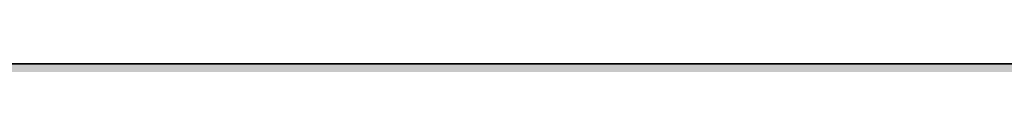
# Model space of a CAD drawing. Units: inches. Extents: x 2091 to 2899, y 967 to 2217.
# Tile 95 of 256: x 2251.5278 to 2251.8124, y 1099.9191 to 1099.9191. Entities that reach past the tile are written whole.
import ezdxf

# ---------------------------------------------------------------- set-up
doc = ezdxf.new("R2010")
doc.units = ezdxf.units.IN
doc.layers.add('A-WALL-PATT', color=141, linetype='Continuous', lineweight=13, true_color=0xadddf7)
doc.layers.add('L-SITE-WALL', color=7, linetype='Continuous', lineweight=35)

msp = doc.modelspace()

# ---------------------------------------------------------------- hatches: boundary and pattern name
at = {"layer": 'A-WALL-PATT'}
h = msp.add_hatch(color=256, dxfattribs=at)
h.dxf.hatch_style = 1
h.paths.add_polyline_path([(2212.1436, 1941.41906), (2387.6436, 1941.41906), (2387.6436, 1824.41906), (2392.1436, 1824.41906), (2392.1436, 1941.41906), (2609.6436, 1941.41906), (2609.6436, 1825.91906), (2614.1436, 1825.91906), (2614.1436, 1941.41906), (2794.1436, 1941.41906), (2794.1436, 1928.76217), (2803.1436, 1928.76217), (2803.1436, 2050.91906), (2203.1436, 2050.91906), (2203.1436, 1900.75786), (2212.1436, 1900.75786)])
h.paths.add_polyline_path([(2212.1436, 1945.91906), (2212.1436, 2041.91906), (2794.1436, 2041.91906), (2794.1436, 1945.91906), (2402.24824, 1945.91906), (2401.10243, 1945.77583), (2398.70243, 1945.77583)], flags=16)
h.paths.add_polyline_path([(2230.22986, 1948.06279), (2227.34986, 1949.50279), (2225.90986, 1951.90279), (2223.98986, 1952.86279), (2223.02986, 1955.26279), (2222.06986, 1959.58279), (2222.06986, 1963.42279), (2223.02986, 1965.66279), (2223.98986, 1965.34279), (2225.58591, 1963.86075), (2226.91153, 1964.95726), (2226.94886, 1965.93879), (2227.77832, 1966.95214), (2228.19992, 1968.8787), (2230.70986, 1964.86279), (2233.58986, 1966.30279), (2233.60731, 1966.33187), (2233.77266, 1964.9382), (2234.6338, 1963.67647), (2235.02986, 1963.90279), (2236.28203, 1965.57236), (2235.98986, 1962.94279), (2237.95451, 1957.54), (2238.38986, 1957.90279), (2239.21586, 1960.30579), (2238.65457, 1966.38496), (2238.69279, 1966.43807), (2238.84058, 1967.49971), (2238.78029, 1967.68749), (2238.88054, 1967.78676), (2238.66686, 1966.25179), (2239.21586, 1960.30579), (2238.38986, 1957.90279), (2236.94986, 1956.70279), (2234.54986, 1949.98279)], flags=0)
h.paths.add_polyline_path([(2278.01197, 1948.06279), (2276.49643, 1947.87335), (2275.84983, 1947.68861), (2274.65197, 1947.10279)], flags=0)
h.paths.add_polyline_path([(2269.85197, 1955.74279), (2268.27618, 1956.62933), (2270.8673, 1956.3484), (2269.37197, 1958.14279), (2268.71496, 1959.19233), (2270.56983, 1958.72861), (2268.58073, 1961.90609), (2270.81197, 1960.89188), (2270.81197, 1963.42279), (2271.39331, 1964.77926), (2270.29176, 1966.1562), (2271.77197, 1965.66279), (2272.14139, 1966.52476), (2273.92983, 1965.92861), (2275.63039, 1968.0543), (2276.33194, 1966.72186), (2276.52043, 1966.95214), (2276.94203, 1968.8787), (2277.73429, 1967.61108), (2278.13989, 1969.46452), (2279.65912, 1967.03374), (2280.41197, 1966.78279), (2280.9493, 1967.58879), (2281.60983, 1967.36861), (2282.13327, 1968.15376), (2282.34924, 1966.33344), (2282.34985, 1966.33259), (2283.40755, 1968.09542), (2283.71263, 1965.52402), (2284.32022, 1964.63379), (2284.51181, 1964.88924), (2284.23497, 1965.70479), (2284.50047, 1967.31896), (2284.90794, 1965.41742), (2285.39631, 1966.06858), (2285.43283, 1966.29061), (2285.47334, 1966.17128), (2286.35392, 1967.34539), (2286.22201, 1966.15817), (2287.66349, 1968.08015), (2287.71397, 1968.44279), (2288.4816, 1969.01668), (2288.57399, 1968.7289), (2288.91746, 1969.06904), (2288.60683, 1966.83761), (2288.92873, 1963.35131), (2288.93497, 1963.35679), (2288.92973, 1963.34042), (2289.01528, 1962.41387), (2290.11122, 1963.87513), (2290.13283, 1963.94261), (2290.21767, 1964.01706), (2290.11122, 1963.87513), (2289.15583, 1960.89161), (2288.59404, 1959.25723), (2288.57197, 1959.10279), (2289.53197, 1960.54279), (2290.01197, 1962.46279), (2290.19184, 1962.64266), (2289.76983, 1959.68861), (2286.88983, 1957.28861), (2284.48983, 1950.56861), (2283.31466, 1950.04631), (2283.29197, 1949.98279), (2280.29006, 1948.64861), (2281.12983, 1948.64861), (2282.56983, 1948.16861), (2283.20473, 1948.06279), (2278.97197, 1948.06279), (2276.09197, 1949.50279), (2274.65197, 1951.90279), (2272.73197, 1952.86279)], flags=0)
h.paths.add_polyline_path([(2271.15887, 1958.02177), (2272.96983, 1955.84861), (2272.00983, 1960.16861), (2272.00983, 1964.00861), (2272.62443, 1965.44266), (2274.32802, 1963.86075), (2275.65365, 1964.95726), (2275.63774, 1964.53909), (2277.41223, 1966.00689), (2277.03297, 1965.15679), (2276.82992, 1964.9756), (2276.76601, 1963.29501), (2277.44964, 1962.66022), (2279.45197, 1964.86279), (2282.33197, 1966.30279), (2283.52983, 1966.88861), (2283.29451, 1966.77095), (2283.91299, 1963.8847), (2284.89925, 1964.44827), (2284.73197, 1962.94279), (2286.69662, 1957.54), (2287.13197, 1957.90279), (2287.54191, 1959.09539), (2287.7794, 1958.44231), (2285.68274, 1956.6951), (2285.8765, 1959.79534), (2284.73197, 1962.94279), (2284.89925, 1964.44827), (2283.91299, 1963.8847), (2284.22383, 1962.43412), (2283.42436, 1963.60548), (2281.60983, 1962.56861), (2281.12983, 1960.16861), (2282.08983, 1956.32861), (2283.04983, 1952.96861), (2282.56983, 1950.56861), (2280.16983, 1948.64861), (2279.88332, 1948.79187), (2278.97197, 1948.06279), (2278.97197, 1949.02279), (2278.67231, 1949.39737), (2277.28983, 1950.08861), (2275.84983, 1952.48861), (2273.92983, 1953.44861), (2272.48983, 1954.88861), (2271.92165, 1954.88861), (2271.77197, 1955.26279)], flags=0)
h.paths.add_polyline_path([(2311.99415, 1955.74279), (2312.06272, 1955.67422), (2312.0551, 1955.7085)], flags=0)
h.paths.add_polyline_path([(2331.95615, 1963.95179), (2333.39615, 1965.39179), (2331.07715, 1963.35679), (2330.9986, 1963.11152)], flags=0)
h.paths.add_polyline_path([(2310.55415, 1954.30279), (2307.03981, 1956.27994), (2310.7629, 1955.87628), (2312.47415, 1953.82279), (2313.43415, 1951.42279), (2315.35415, 1950.46279), (2316.79415, 1948.06279), (2317.46615, 1947.72679), (2319.36869, 1947.96461), (2317.75415, 1949.98279), (2317.56953, 1950.61048), (2316.79415, 1951.90279), (2314.87415, 1952.86279), (2313.91415, 1955.26279), (2311.51415, 1958.14279), (2309.37549, 1961.55917), (2311.51415, 1960.33708), (2311.51415, 1961.98279), (2310.60467, 1963.11963), (2311.72661, 1962.47853), (2312.41833, 1964.09256), (2312.25596, 1964.29552), (2313.19415, 1963.98279), (2313.91415, 1965.66279), (2314.64678, 1965.41858), (2315.35415, 1966.30279), (2316.79415, 1967.74279), (2316.15744, 1966.9469), (2317.03411, 1965.28186), (2317.2226, 1965.51214), (2317.77705, 1968.04577), (2318.47411, 1966.72186), (2318.6626, 1966.95214), (2319.0842, 1968.8787), (2321.20705, 1965.48215), (2322.16142, 1966.9137), (2322.55415, 1966.78279), (2322.78599, 1967.13056), (2322.88165, 1966.32429), (2323.31204, 1965.72174), (2323.65129, 1965.89136), (2324.3965, 1967.13338), (2324.65694, 1964.9382), (2324.97199, 1964.47661), (2325.38728, 1967.0015), (2325.94081, 1964.41835), (2327.22893, 1966.13584), (2327.16632, 1965.57236), (2328.05914, 1966.76278), (2328.22458, 1966.24749), (2329.66797, 1967.67691), (2329.66458, 1967.68749), (2329.76482, 1967.78676), (2329.55115, 1966.25179), (2330.10015, 1960.30579), (2329.33281, 1958.07347), (2329.31306, 1957.93523), (2329.63415, 1958.20279), (2330.23415, 1959.10279), (2330.71415, 1961.02279), (2331.03415, 1961.34279), (2330.71415, 1959.10279), (2329.63415, 1958.20279), (2329.27415, 1957.66279), (2327.71211, 1956.3611), (2325.43415, 1949.98279), (2324.33377, 1949.49374), (2323.99415, 1948.54279), (2319.67415, 1946.62279), (2316.79415, 1948.06279), (2315.35415, 1950.46279), (2313.43415, 1951.42279)], flags=0)
h.paths.add_polyline_path([(2321.33568, 1947.95202), (2321.11415, 1948.06279), (2321.11415, 1949.02279), (2319.19415, 1951.42279), (2316.79415, 1959.58279), (2316.66324, 1959.58279), (2315.35415, 1958.14279), (2314.39415, 1958.14279), (2313.1483, 1958.70908), (2312.95415, 1959.58279), (2312.95415, 1960.89188), (2315.83415, 1959.58279), (2316.66324, 1959.58279), (2317.31471, 1960.29941), (2315.0302, 1962.42075), (2316.35582, 1963.51726), (2316.37234, 1963.95162), (2316.4702, 1963.86075), (2317.79582, 1964.95726), (2317.75522, 1963.88969), (2319.17515, 1965.15679), (2319.49841, 1965.88137), (2321.11415, 1965.34279), (2323.23589, 1962.37236), (2325.68635, 1963.77262), (2325.54279, 1962.48058), (2325.19878, 1963.49401), (2324.47851, 1963.08243), (2324.92601, 1960.99412), (2324.07809, 1962.23647), (2322.41479, 1961.28602), (2322.07415, 1959.58279), (2323.03415, 1955.74279), (2323.99415, 1952.38279), (2323.51415, 1949.98279), (2322.14272, 1948.88565), (2322.07415, 1948.54279)], flags=0)
h.paths.add_polyline_path([(2320.20748, 1963.33746), (2320.15415, 1963.42279), (2320.39415, 1963.54279)], flags=0)
h.paths.add_polyline_path([(2353.85053, 1965.8105), (2354.03053, 1965.7505), (2354.33053, 1966.4505), (2354.33053, 1966.9305)], flags=0)
h.paths.add_polyline_path([(2359.02058, 1969.02641), (2359.09838, 1968.90193), (2359.23353, 1969.5195), (2359.23353, 1969.9995)], flags=0)
h.paths.add_polyline_path([(2358.25669, 1966.68167), (2357.9836, 1966.34803), (2358.21127, 1966.14617), (2358.41049, 1966.38957)], flags=0)
h.paths.add_polyline_path([(2357.76847, 1966.05878), (2357.7322, 1965.10497), (2357.75105, 1965.12056), (2357.76953, 1965.6065), (2357.76953, 1966.05784)], flags=0)
h.paths.add_polyline_path([(2359.11153, 1965.3045), (2359.11153, 1964.8245), (2359.84453, 1966.4675), (2359.84453, 1966.9475)], flags=0)
h.paths.add_polyline_path([(2360.22368, 1966.62145), (2360.69853, 1969.3625), (2360.69853, 1969.8425), (2360.21053, 1967.0255), (2360.21053, 1966.6425)], flags=0)
h.paths.add_polyline_path([(2363.45053, 1967.8905), (2363.45053, 1968.3705), (2362.49053, 1966.9305), (2362.65604, 1966.69878)], flags=0)
h.paths.add_polyline_path([(2364.47552, 1966.07883), (2365.85053, 1968.3705), (2365.85053, 1968.8505), (2364.42798, 1966.47958)], flags=0)
h.paths.add_polyline_path([(2366.31353, 1965.8525), (2366.36671, 1965.69583), (2366.80253, 1968.3455), (2366.80253, 1968.8255)], flags=0)
h.paths.add_polyline_path([(2367.16531, 1965.80354), (2367.29053, 1966.9305), (2367.29053, 1967.4105), (2367.1027, 1965.72007)], flags=0)
h.paths.add_polyline_path([(2370.03653, 1959.9735), (2371.01353, 1963.0245), (2371.01353, 1963.5045), (2370.03653, 1960.4535)], flags=0)
h.paths.add_polyline_path([(2371.61053, 1960.2105), (2372.57053, 1961.6505), (2372.57053, 1962.1305), (2371.80253, 1960.9785)], flags=0)
h.paths.add_polyline_path([(2350.87367, 1956.00509), (2351.93053, 1955.8905), (2354.49053, 1953.3305), (2353.85053, 1954.9305), (2351.45053, 1957.8105), (2347.93553, 1963.4255), (2347.93553, 1963.9055), (2351.45053, 1958.2905), (2353.70507, 1955.58505), (2352.89053, 1959.2505), (2352.89053, 1959.7305), (2352.89053, 1961.92479), (2356.73053, 1959.7305), (2358.45447, 1961.62684), (2354.81053, 1965.0105), (2355.03086, 1965.28591), (2358.69109, 1961.88712), (2361.53053, 1965.0105), (2364.3765, 1966.43348), (2364.52439, 1965.18691), (2365.45447, 1963.82418), (2365.88107, 1964.06795), (2365.37053, 1966.4505), (2365.37053, 1966.9305), (2366.81053, 1960.2105), (2366.81053, 1959.7305), (2366.38871, 1952.98141), (2367.77053, 1956.8505), (2368.64123, 1957.57608), (2366.81053, 1962.6105), (2366.81053, 1963.0905), (2368.77518, 1957.68771), (2369.21053, 1958.0505), (2370.00159, 1960.35187), (2369.47523, 1966.05267), (2369.51346, 1966.10578), (2369.51417, 1966.11091), (2369.47523, 1966.53267), (2369.51346, 1966.58578), (2369.61463, 1967.31259), (2369.18253, 1968.6585), (2369.18253, 1969.1385), (2369.60096, 1967.83519), (2369.7012, 1967.93447), (2369.71795, 1968.05474), (2370.14518, 1968.37414), (2369.77871, 1968.01122), (2369.7012, 1967.45447), (2370.46816, 1968.214), (2369.67494, 1967.26577), (2369.51417, 1966.11091), (2370.03653, 1960.4535), (2370.03653, 1959.9735), (2369.44176, 1958.24319), (2370.65053, 1959.2505), (2371.04582, 1962.01756), (2371.13053, 1962.1305), (2370.65053, 1958.7705), (2367.77053, 1956.3705), (2365.37053, 1949.6505), (2362.0791, 1948.18764), (2363.45053, 1947.7305), (2361.05053, 1947.7305), (2360.09053, 1947.7305), (2357.10386, 1947.35717), (2360.09053, 1948.2105), (2358.17053, 1949.1705), (2356.73053, 1951.5705), (2354.81053, 1952.5305), (2351.93053, 1955.4105)], flags=0)
h.paths.add_polyline_path([(2361.05053, 1948.6905), (2359.13053, 1951.0905), (2356.73053, 1959.2505), (2355.77053, 1959.2505), (2352.89053, 1960.55959), (2352.89053, 1961.44479), (2355.89053, 1959.7305), (2356.73053, 1959.7305), (2356.83719, 1959.36783), (2361.53053, 1964.5305), (2363.24842, 1965.38945), (2364.92531, 1963.0418), (2362.49053, 1961.6505), (2362.06386, 1959.51717), (2362.97053, 1955.8905), (2363.93053, 1952.5305), (2363.93053, 1952.0505), (2363.45053, 1949.6505), (2361.05053, 1947.7305)], flags=0)
h.paths.add_polyline_path([(2359.13053, 1951.5705), (2359.29053, 1951.3705), (2361.05053, 1954.4505), (2361.05053, 1954.9305)], flags=0)
h.paths.add_polyline_path([(2357.21953, 1966.5455), (2356.79253, 1968.8145), (2356.79253, 1969.2945), (2357.21953, 1967.0255)], flags=0)
h.paths.add_polyline_path([(2361.05053, 1954.4505), (2361.53053, 1958.7705), (2361.53053, 1959.2505), (2361.05053, 1954.9305)], flags=0)
h.paths.add_polyline_path([(2402.54829, 1948.48608), (2402.30243, 1948.41583), (2402.59043, 1948.41583)], flags=0)
h.paths.add_polyline_path([(2394.14243, 1956.09583), (2395.68505, 1954.55321), (2396.7205, 1953.97068), (2396.06243, 1955.61583), (2395.24138, 1956.6011), (2395.8789, 1956.44171), (2395.10243, 1959.93583), (2395.10243, 1963.77583), (2396.06243, 1966.01583), (2397.02243, 1965.69583), (2398.61848, 1964.21379), (2399.94411, 1965.3103), (2399.98143, 1966.29183), (2400.81089, 1967.30518), (2401.23249, 1969.23174), (2403.53795, 1965.54301), (2403.94198, 1967.38932), (2404.70243, 1967.13583), (2405.46033, 1966.07478), (2406.62243, 1966.65583), (2406.63988, 1966.68491), (2406.80523, 1965.29124), (2406.92569, 1965.11475), (2407.34243, 1964.97583), (2407.87433, 1965.77367), (2408.1691, 1964.39805), (2409.31461, 1965.9254), (2409.21746, 1965.05105), (2409.44523, 1963.13124), (2410.30637, 1961.86951), (2410.70243, 1962.09583), (2411.44227, 1963.08228), (2411.16543, 1963.89783), (2411.61643, 1966.63976), (2411.72536, 1966.79111), (2411.87315, 1967.85275), (2411.81286, 1968.04053), (2411.91311, 1968.1398), (2411.69943, 1966.60483), (2412.24843, 1960.65883), (2413.22543, 1963.70983), (2414.3779, 1964.72116), (2414.51315, 1965.69275), (2414.45286, 1965.88053), (2414.55311, 1965.9798), (2414.3779, 1964.72116), (2414.51982, 1964.8457), (2414.36536, 1964.63111), (2414.33943, 1964.44483), (2414.88843, 1958.49883), (2414.06243, 1956.09583), (2412.62243, 1954.89583), (2410.17137, 1948.03285), (2410.01672, 1948.0844), (2405.90243, 1946.25583), (2405.90243, 1947.21583), (2405.20425, 1948.08856), (2404.22243, 1948.41583), (2403.26243, 1948.41583), (2400.38243, 1949.85583), (2399.66243, 1951.05583), (2397.98243, 1952.73583), (2397.02243, 1953.21583), (2395.68505, 1954.55321), (2392.65678, 1956.25691)], flags=0)
h.paths.add_polyline_path([(2409.08565, 1964.40744), (2409.13036, 1964.27572), (2409.26243, 1964.49583)], flags=0)
h.paths.add_polyline_path([(2397.74243, 1961.61583), (2398.70243, 1963.85583), (2399.66243, 1963.53583), (2401.42656, 1965.74099), (2401.79142, 1966.5588), (2402.07143, 1965.07083), (2402.83551, 1964.39337), (2403.2624, 1964.9149), (2403.33812, 1964.77109), (2402.61552, 1963.97622), (2402.49861, 1960.90224), (2403.543, 1959.93245), (2404.4132, 1960.88968), (2404.70243, 1962.33583), (2407.91635, 1964.17235), (2409.52021, 1961.92694), (2410.98708, 1957.89304), (2411.42243, 1958.25583), (2412.04796, 1960.07562), (2412.41034, 1959.07909), (2411.67562, 1958.46682), (2411.66243, 1958.25583), (2411.62607, 1958.42553), (2409.98243, 1957.05583), (2407.58243, 1950.33583), (2403.26243, 1948.41583), (2403.26243, 1949.37583), (2401.34243, 1951.77583), (2399.41651, 1958.32398), (2397.74243, 1959.08492), (2397.74243, 1959.97012), (2397.10243, 1960.33583), (2397.74243, 1960.04492)], flags=0)
h.paths.add_polyline_path([(2405.90243, 1952.97583), (2405.95043, 1953.40783), (2406.01672, 1953.17583)], flags=0)
h.paths.add_polyline_path([(2449.81778, 1967.11401), (2449.75232, 1967.13583), (2449.7937, 1967.0779)], flags=0)
h.paths.add_polyline_path([(2451.6977, 1966.61812), (2451.74089, 1966.69012), (2451.69205, 1966.6657)], flags=0)
h.paths.add_polyline_path([(2454.34363, 1965.73757), (2455.75232, 1967.61583), (2455.99232, 1968.09583), (2454.3645, 1965.9254)], flags=0)
h.paths.add_polyline_path([(2457.54732, 1968.86383), (2457.78732, 1969.34383), (2457.05432, 1968.79583), (2457.00762, 1968.46034)], flags=0)
h.paths.add_polyline_path([(2456.92178, 1967.85666), (2456.80224, 1968.22902), (2456.723, 1967.6598)], flags=0)
h.paths.add_polyline_path([(2457.30232, 1967.37683), (2457.54232, 1967.85683), (2456.81032, 1966.83983), (2456.74052, 1966.70022), (2456.74902, 1966.60811)], flags=0)
h.paths.add_polyline_path([(2458.27532, 1963.70983), (2458.15534, 1963.33515), (2460.35432, 1965.26483), (2460.59432, 1965.74483)], flags=0)
h.paths.add_polyline_path([(2458.39232, 1962.81583), (2458.36409, 1962.61819), (2459.59232, 1964.25583), (2459.83232, 1964.73583)], flags=0)
h.paths.add_polyline_path([(2459.35232, 1962.81583), (2459.27232, 1962.49583), (2460.07232, 1963.29583), (2460.31232, 1963.77583)], flags=0)
h.paths.add_polyline_path([(2458.68032, 1960.60783), (2458.63232, 1960.41583), (2459.59232, 1961.85583), (2459.83232, 1962.33583)], flags=0)
h.paths.add_polyline_path([(2437.83817, 1956.24265), (2439.19232, 1956.09583), (2441.35232, 1953.93583), (2440.87232, 1955.13583), (2438.47232, 1958.01583), (2438.07156, 1958.65602), (2438.71232, 1958.49583), (2440.6396, 1956.18311), (2439.91232, 1959.45583), (2439.91232, 1963.29583), (2441.35232, 1966.65583), (2441.59232, 1967.13583), (2441.11232, 1966.01583), (2442.07232, 1965.69583), (2443.98899, 1968.09167), (2444.24132, 1966.75083), (2444.9168, 1966.15192), (2445.67657, 1967.08014), (2446.25532, 1969.72483), (2446.49532, 1970.20483), (2446.28238, 1969.23174), (2447.36267, 1967.50327), (2447.72032, 1969.56783), (2447.96032, 1970.04783), (2447.48548, 1967.30678), (2448.79232, 1965.21583), (2448.47232, 1964.86383), (2448.55232, 1964.73583), (2451.45205, 1966.1857), (2451.61512, 1964.81124), (2452.30792, 1963.79617), (2453.23451, 1964.32565), (2454.07232, 1960.41583), (2453.62869, 1953.31765), (2454.79232, 1956.57583), (2455.03232, 1957.05583), (2455.71884, 1957.62793), (2453.83232, 1962.81583), (2453.94097, 1963.79362), (2453.33532, 1965.57783), (2453.82432, 1968.55083), (2454.06432, 1969.03083), (2453.57532, 1966.05783), (2454.04033, 1964.68792), (2453.83232, 1962.81583), (2455.71884, 1957.62793), (2456.36721, 1958.16824), (2457.05832, 1960.17883), (2457.29832, 1960.65883), (2456.47232, 1958.25583), (2457.71773, 1959.29367), (2457.67232, 1958.97583), (2454.88995, 1956.65719), (2453.61414, 1953.08492), (2453.59232, 1952.73583), (2453.35232, 1952.25583), (2453.3596, 1952.3722), (2452.63232, 1950.33583), (2452.39232, 1949.85583), (2449.20375, 1948.43869), (2450.71232, 1947.93583), (2448.07232, 1947.93583), (2447.11232, 1947.93583), (2444.55232, 1947.61583), (2447.1996, 1948.3722), (2445.19232, 1949.37583), (2443.75232, 1951.77583), (2441.83232, 1952.73583), (2438.95232, 1955.61583)], flags=0)
h.paths.add_polyline_path([(2443.99232, 1959.93583), (2444.04032, 1959.77263), (2444.12155, 1959.86199)], flags=0)
h.paths.add_polyline_path([(2442.91232, 1959.93583), (2443.03232, 1959.93583), (2442.44566, 1960.2025)], flags=0)
h.paths.add_polyline_path([(2444.98294, 1965.01968), (2445.27932, 1965.26483), (2445.51932, 1965.74483), (2444.994, 1965.3103)], flags=0)
h.paths.add_polyline_path([(2446.13332, 1965.02983), (2446.33037, 1965.4715), (2444.97032, 1964.25783), (2444.73032, 1963.77783)], flags=0)
h.paths.add_polyline_path([(2442.79232, 1959.45583), (2443.75232, 1959.45583), (2446.15232, 1951.29583), (2446.41232, 1951.75083), (2446.39232, 1951.77583), (2448.0806, 1954.73032), (2448.55232, 1958.97583), (2441.83232, 1965.21583), (2442.15495, 1965.61911), (2448.79232, 1959.45583), (2448.31232, 1955.13583), (2448.07232, 1954.65583), (2446.41232, 1951.75083), (2448.31232, 1949.37583), (2448.31232, 1948.41583), (2450.54089, 1950.19869), (2450.95232, 1952.25583), (2449.99232, 1955.61583), (2449.03232, 1959.45583), (2449.51232, 1961.85583), (2449.75232, 1962.33583), (2449.6749, 1961.94874), (2452.99451, 1963.84565), (2453.06441, 1963.51941), (2452.88461, 1963.78285), (2449.6749, 1961.94874), (2449.27232, 1959.93583), (2450.23232, 1956.09583), (2451.19232, 1952.73583), (2450.71232, 1950.33583), (2450.47232, 1949.85583), (2448.07232, 1947.93583), (2448.07232, 1948.53583), (2445.43232, 1949.85583), (2443.99232, 1952.25583), (2442.07232, 1953.21583), (2441.11232, 1955.61583), (2440.15232, 1959.93583), (2440.15232, 1960.65583)], flags=0)
h.paths.add_polyline_path([(2456.69232, 1966.98583), (2457.60832, 1968.08083), (2457.84832, 1968.56083), (2456.93232, 1967.46583)], flags=0)
h.paths.add_polyline_path([(2489.89657, 1966.58024), (2489.94295, 1966.18935), (2490.74749, 1967.53025), (2491.31912, 1968.95116)], flags=0)
h.paths.add_polyline_path([(2473.56247, 1956.40713), (2477.13998, 1956.01926), (2476.95533, 1956.24083), (2475.10805, 1957.28011), (2476.34749, 1956.97025), (2475.1869, 1958.82422), (2476.91912, 1958.39116), (2475.41164, 1960.79927), (2477.78749, 1959.71934), (2477.78749, 1962.25025), (2477.6374, 1962.43786), (2477.82255, 1962.33206), (2478.35912, 1963.58406), (2478.35912, 1963.67116), (2477.32435, 1964.96463), (2478.71483, 1964.50114), (2479.31912, 1965.91116), (2480.27912, 1965.59116), (2481.78397, 1967.47221), (2482.11649, 1965.70525), (2482.88056, 1965.02778), (2483.20931, 1965.42941), (2483.22017, 1965.71509), (2483.07594, 1965.98902), (2483.71176, 1966.76581), (2484.13049, 1968.67925), (2484.70212, 1970.10016), (2484.48918, 1969.12707), (2486.5029, 1965.90511), (2487.38749, 1965.61025), (2488.15342, 1966.75914), (2488.71702, 1965.97011), (2489.20009, 1966.21164), (2489.33067, 1965.11099), (2490.3939, 1963.62246), (2490.66077, 1963.77496), (2490.49391, 1964.55364), (2490.92306, 1963.92484), (2491.31912, 1964.15116), (2491.33339, 1964.17018), (2491.21049, 1964.53225), (2491.28176, 1964.96554), (2491.42579, 1964.29338), (2494.07648, 1967.82763), (2494.49792, 1966.51494), (2494.59817, 1966.61422), (2494.68949, 1967.27025), (2495.10675, 1967.5822), (2495.12984, 1967.74807), (2495.06955, 1967.93585), (2495.1698, 1968.03513), (2495.03178, 1967.04363), (2495.75382, 1967.75868), (2494.98205, 1966.68644), (2494.95612, 1966.50016), (2495.47902, 1960.83685), (2495.91049, 1962.18425), (2496.48212, 1963.60516), (2496.07269, 1962.32659), (2496.7689, 1962.93754), (2496.59912, 1962.71116), (2496.11912, 1959.35116), (2496.73287, 1960.27179), (2496.98749, 1961.29025), (2497.55912, 1962.71116), (2497.07912, 1960.79116), (2496.50749, 1959.37025), (2495.54749, 1957.93025), (2492.75884, 1955.60638), (2490.83912, 1950.23116), (2490.26749, 1948.81025), (2485.94749, 1946.89025), (2483.06749, 1948.33025), (2481.62749, 1950.73025), (2479.70749, 1951.69025), (2476.82749, 1954.57025)], flags=0)
h.paths.add_polyline_path([(2485.57697, 1948.31339), (2485.55912, 1948.31116), (2485.57876, 1948.31116)], flags=0)
h.paths.add_polyline_path([(2478.64506, 1954.55116), (2478.10904, 1956.96326), (2479.31912, 1955.51116), (2480.27912, 1953.11116), (2482.19912, 1952.15116), (2483.63912, 1949.75116), (2486.51912, 1948.31116), (2486.51912, 1949.27116), (2484.73931, 1951.49593), (2484.02749, 1950.25025), (2481.62749, 1958.41025), (2482.37515, 1959.23267), (2482.19912, 1959.83116), (2483.19757, 1960.92946), (2479.70749, 1964.17025), (2480.60336, 1965.29008), (2481.87517, 1964.10911), (2482.66639, 1964.76358), (2482.61536, 1963.4218), (2482.9892, 1963.07466), (2484.00849, 1963.98425), (2484.68361, 1965.49751), (2484.58012, 1965.40516), (2485.35727, 1967.14711), (2485.12065, 1965.7812), (2486.42749, 1963.69025), (2488.14538, 1964.5492), (2489.82227, 1962.20155), (2490.74749, 1962.73025), (2491.99966, 1964.39981), (2492.07605, 1965.08726), (2492.21289, 1964.68412), (2492.48537, 1965.04743), (2492.27912, 1963.19116), (2494.24377, 1957.78837), (2494.5625, 1958.05398), (2494.93349, 1959.13325), (2495.50512, 1960.55416), (2494.67912, 1958.15116), (2494.10749, 1956.73025), (2494.5625, 1958.05398), (2493.40854, 1957.09235), (2491.70749, 1961.77025), (2491.99966, 1964.39981), (2490.74749, 1962.73025), (2487.71203, 1960.9957), (2487.47912, 1959.83116), (2488.43912, 1955.99116), (2489.39912, 1952.63116), (2488.91912, 1950.23116), (2488.57692, 1949.9574), (2488.34749, 1948.81025), (2487.65172, 1948.25363), (2487.47912, 1948.31116), (2486.51912, 1948.31116), (2483.63912, 1949.75116), (2482.19912, 1952.15116), (2480.27912, 1953.11116), (2478.83912, 1954.55116)], flags=0)
h.paths.add_polyline_path([(2526.64825, 1966.98752), (2526.51734, 1967.03116), (2526.6001, 1966.9153)], flags=0)
h.paths.add_polyline_path([(2528.47064, 1966.44666), (2528.57449, 1966.61973), (2528.45707, 1966.56102)], flags=0)
h.paths.add_polyline_path([(2534.13334, 1967.49616), (2534.15669, 1967.54285), (2534.05984, 1967.4083)], flags=0)
h.paths.add_polyline_path([(2536.16192, 1964.0506), (2535.15734, 1962.71116), (2535.10087, 1962.31587), (2536.11734, 1963.67116), (2536.42053, 1964.27754)], flags=0)
h.paths.add_polyline_path([(2535.15734, 1959.83116), (2536.11734, 1961.27116), (2536.59734, 1962.23116), (2535.25334, 1960.21516)], flags=0)
h.paths.add_polyline_path([(2513.24904, 1956.2848), (2516.22118, 1955.96256), (2514.99734, 1957.43116), (2514.19582, 1958.71154), (2515.47734, 1958.39116), (2516.93189, 1956.64571), (2516.43734, 1958.87116), (2516.43734, 1962.71116), (2516.87269, 1963.72697), (2515.34643, 1965.6348), (2517.39734, 1964.95116), (2517.87734, 1966.07116), (2518.35734, 1967.03116), (2517.87734, 1965.91116), (2518.83734, 1965.59116), (2520.48659, 1967.65272), (2520.76634, 1966.16616), (2521.53042, 1965.48869), (2521.78144, 1965.79537), (2521.80091, 1966.30727), (2521.4778, 1966.92094), (2521.24634, 1967.12616), (2521.1777, 1967.49091), (2521.4778, 1966.92094), (2522.01042, 1966.44869), (2522.25739, 1966.75042), (2522.78034, 1969.14016), (2523.26034, 1970.10016), (2523.0474, 1969.12707), (2524.67313, 1966.5259), (2526.03734, 1966.07116), (2526.79524, 1965.01011), (2527.97707, 1965.60102), (2528.14014, 1964.22657), (2528.66459, 1963.45816), (2529.38862, 1963.87189), (2529.32967, 1964.14699), (2529.48128, 1963.92484), (2529.87734, 1964.15116), (2529.98401, 1964.29338), (2529.78905, 1965.20318), (2530.0624, 1964.3979), (2532.80248, 1968.05135), (2533.14777, 1966.97585), (2533.24802, 1967.07513), (2533.33934, 1967.73116), (2533.67285, 1967.98049), (2533.72802, 1968.03513), (2533.51434, 1966.50016), (2534.02472, 1960.9725), (2534.56034, 1962.64516), (2535.04034, 1963.60516), (2534.06334, 1960.55416), (2533.23734, 1958.15116), (2534.28815, 1959.02684), (2534.19734, 1958.39116), (2531.5126, 1956.15387), (2529.39734, 1950.23116), (2528.91734, 1949.27116), (2526.44877, 1948.17402), (2527.47734, 1947.83116), (2530.35734, 1947.35116), (2524.59734, 1947.35116), (2521.71734, 1948.79116), (2520.27734, 1951.19116), (2518.35734, 1952.15116), (2515.47734, 1955.03116)], flags=0)
h.paths.add_polyline_path([(2523.93476, 1967.19031), (2523.61951, 1966.48369), (2523.7705, 1966.24211)], flags=0)
h.paths.add_polyline_path([(2518.83734, 1953.11116), (2517.87734, 1955.51116), (2516.88498, 1959.97678), (2516.91734, 1959.96207), (2516.91734, 1962.02545), (2520.75734, 1959.83116), (2522.02495, 1961.22553), (2518.35734, 1964.63116), (2519.00259, 1965.43772), (2520.43339, 1964.10911), (2521.30112, 1964.82687), (2521.24516, 1963.35533), (2525.63831, 1959.27598), (2526.03734, 1961.27116), (2529.39734, 1963.19116), (2530.64952, 1964.86073), (2530.66472, 1964.99755), (2530.69196, 1964.91731), (2531.08778, 1965.44507), (2530.94599, 1964.16894), (2530.69196, 1964.91731), (2529.39734, 1963.19116), (2526.3625, 1961.45697), (2526.03734, 1959.83116), (2526.99734, 1955.99116), (2527.95734, 1952.63116), (2527.47734, 1950.23116), (2527.13449, 1949.95687), (2526.97393, 1949.15409), (2526.69734, 1949.03116), (2524.59734, 1947.35116), (2524.59734, 1948.31116), (2524.27734, 1948.71116), (2522.19734, 1949.75116), (2520.75734, 1952.15116)], flags=0)
h.paths.add_polyline_path([(2520.27734, 1958.87116), (2520.85334, 1959.50476), (2523.15734, 1951.67116), (2524.61389, 1954.22013), (2524.59734, 1954.07116), (2522.67734, 1950.71116)], flags=0)
h.paths.add_polyline_path([(2559.37091, 1966.31116), (2559.39841, 1966.32491), (2559.40194, 1966.3453)], flags=0)
h.paths.add_polyline_path([(2549.77091, 1957.19116), (2552.65091, 1954.31116), (2552.13399, 1955.60347), (2550.61091, 1957.43116), (2547.09591, 1963.04616), (2545.77591, 1965.20616), (2549.29091, 1959.59116), (2551.69091, 1956.71116), (2550.79293, 1960.75206), (2550.73091, 1960.78025), (2550.73091, 1964.87116), (2551.69091, 1967.11116), (2552.65091, 1966.79116), (2554.24696, 1965.30911), (2555.03425, 1965.96034), (2555.58167, 1966.64461), (2555.60991, 1967.38716), (2556.43937, 1968.40051), (2556.86097, 1970.32707), (2559.37091, 1966.31116), (2560.69091, 1964.15116), (2562.40881, 1965.01011), (2561.65091, 1966.07116), (2560.33091, 1968.23116), (2561.7585, 1966.23254), (2562.34721, 1967.11561), (2562.43371, 1966.38657), (2563.1278, 1965.3696), (2563.57091, 1965.59116), (2563.58836, 1965.62024), (2563.36254, 1967.52354), (2563.72249, 1965.84379), (2565.06, 1968.07298), (2564.73286, 1965.12872), (2565.11758, 1963.33338), (2567.44462, 1966.43611), (2567.31561, 1967.83333), (2567.35384, 1967.88644), (2567.50163, 1968.94807), (2567.44134, 1969.13585), (2567.54159, 1969.23513), (2567.32791, 1967.70016), (2567.87691, 1961.75416), (2568.74669, 1964.47033), (2568.63561, 1965.67333), (2568.67384, 1965.72644), (2568.82163, 1966.78807), (2568.76134, 1966.97585), (2568.86159, 1967.07513), (2568.64791, 1965.54016), (2568.72613, 1964.69303), (2568.85391, 1964.80516), (2568.74669, 1964.47033), (2568.81724, 1963.70626), (2568.97091, 1963.91116), (2568.86607, 1963.17731), (2569.19691, 1959.59416), (2568.37091, 1957.19116), (2566.93091, 1955.99116), (2564.62027, 1949.52137), (2564.65091, 1949.51116), (2564.61662, 1949.51116), (2564.53091, 1949.27116), (2560.21091, 1947.35116), (2557.33091, 1948.79116), (2556.0452, 1950.93402), (2556.01091, 1950.95116), (2555.85662, 1951.2083), (2553.97091, 1952.15116), (2551.09091, 1955.03116), (2546.65014, 1957.52951)], flags=0)
h.paths.add_polyline_path([(2567.02579, 1959.33023), (2567.03501, 1959.30489), (2567.05091, 1959.35116)], flags=0)
h.paths.add_polyline_path([(2551.96829, 1962.51837), (2553.01091, 1964.95116), (2553.97091, 1964.63116), (2555.56696, 1963.14911), (2556.89258, 1964.24563), (2556.92991, 1965.22716), (2557.14398, 1965.48869), (2556.42007, 1966.13056), (2556.39142, 1966.10499), (2556.37991, 1966.16616), (2556.42007, 1966.13056), (2556.95191, 1966.60516), (2557.09214, 1966.91948), (2557.57087, 1966.01023), (2557.75937, 1966.24051), (2557.41791, 1964.68016), (2556.89258, 1964.24563), (2556.80709, 1961.99757), (2560.69091, 1958.39116), (2560.63553, 1957.8927), (2560.81091, 1957.19116), (2561.77091, 1953.83116), (2561.29091, 1951.43116), (2559.11042, 1949.68677), (2559.15648, 1949.62919), (2563.02652, 1951.34921), (2562.61091, 1949.27116), (2560.21091, 1947.35116), (2560.21091, 1948.31116), (2559.25091, 1949.51116), (2558.89091, 1949.51116), (2558.89091, 1949.96116), (2558.29091, 1950.71116), (2558.0537, 1951.51767), (2556.97091, 1952.87116), (2555.06788, 1959.34146), (2552.05091, 1961.06545), (2552.05091, 1962.47116)], flags=0)
h.paths.add_polyline_path([(2588.33005, 1958.39116), (2588.61025, 1958.11096), (2588.55336, 1958.36695)], flags=0)
h.paths.add_polyline_path([(2594.74545, 1950.49309), (2593.95753, 1953.17202), (2593.13005, 1954.55116), (2591.21005, 1955.51116), (2590.25005, 1957.91116), (2588.30903, 1960.24038), (2586.17731, 1961.20935), (2587.85005, 1960.79116), (2587.25342, 1961.74425), (2588.44131, 1961.06545), (2588.44131, 1962.65553), (2588.42168, 1962.66535), (2588.44131, 1962.71116), (2586.91404, 1964.62026), (2588.87709, 1963.72796), (2589.29005, 1964.69154), (2589.29005, 1966.07116), (2590.25005, 1968.31116), (2591.21005, 1967.99116), (2592.8061, 1966.50911), (2594.13172, 1967.60563), (2594.16905, 1968.58716), (2594.99851, 1969.60051), (2595.4201, 1971.52707), (2597.93005, 1967.51116), (2600.81005, 1968.95116), (2600.8275, 1968.98024), (2600.99285, 1967.58657), (2601.85399, 1966.32484), (2602.10714, 1966.4695), (2602.23635, 1967.25507), (2602.35672, 1966.69338), (2603.50222, 1968.22073), (2603.21005, 1965.59116), (2605.1747, 1960.18837), (2605.50689, 1960.4652), (2605.02602, 1965.67333), (2605.06425, 1965.72644), (2605.21203, 1966.78807), (2605.15174, 1966.97585), (2605.25199, 1967.07513), (2605.34331, 1967.73116), (2605.9529, 1968.1869), (2605.87475, 1969.03333), (2605.91298, 1969.08644), (2606.06077, 1970.14807), (2606.00048, 1970.33585), (2606.10073, 1970.43513), (2605.88705, 1968.90016), (2606.43605, 1962.95416), (2605.61005, 1960.55116), (2605.99704, 1960.87365), (2606.56431, 1962.64516), (2608.24149, 1964.11694), (2608.01005, 1963.19116), (2607.05005, 1961.75116), (2606.63149, 1961.40236), (2606.20131, 1958.39116), (2603.32131, 1955.99116), (2600.92131, 1949.27116), (2596.60131, 1947.35116), (2593.72131, 1948.79116), (2592.85731, 1950.23116), (2592.65005, 1950.23116)], flags=0)
h.paths.add_polyline_path([(2596.60131, 1947.35116), (2596.60131, 1948.31116), (2594.68131, 1950.71116), (2596.15495, 1953.29003), (2595.53005, 1954.07116), (2593.19923, 1961.99596), (2592.65134, 1962.50471), (2591.78015, 1963.00253), (2593.28299, 1964.24563), (2593.32031, 1965.22716), (2594.14977, 1966.24051), (2594.57137, 1968.16707), (2596.18265, 1965.58902), (2596.95127, 1966.43451), (2598.04131, 1966.07116), (2598.79921, 1965.01011), (2599.96131, 1965.59116), (2599.97876, 1965.62024), (2600.14411, 1964.22657), (2601.00526, 1962.96484), (2601.40131, 1963.19116), (2602.65349, 1964.86073), (2602.36131, 1962.23116), (2603.79275, 1958.29472), (2601.97764, 1953.21243), (2601.94621, 1952.70945), (2599.46876, 1951.60836), (2599.00131, 1949.27116)], flags=0)
h.paths.add_polyline_path([(2597.56131, 1958.87116), (2597.67097, 1959.41942), (2597.59505, 1958.7362)], flags=0)
h.paths.add_polyline_path([(2623.6663, 1961.25438), (2625.51916, 1960.79116), (2624.96554, 1961.67553), (2627.19916, 1960.66025), (2627.19916, 1961.15116), (2626.95916, 1962.23116), (2626.95916, 1963.49116), (2625.58232, 1965.21221), (2626.95916, 1964.42545), (2626.95916, 1965.83116), (2626.86916, 1965.86116), (2627.91916, 1968.31116), (2628.87916, 1967.99116), (2630.47521, 1966.50911), (2631.80084, 1967.60563), (2631.83816, 1968.58716), (2632.66762, 1969.60051), (2633.08922, 1971.52707), (2635.59916, 1967.51116), (2638.47916, 1968.95116), (2638.49661, 1968.98024), (2638.66196, 1967.58657), (2639.17627, 1966.83301), (2639.78022, 1967.83958), (2640.02583, 1966.69338), (2641.17134, 1968.22073), (2640.87916, 1965.59116), (2641.11426, 1964.94463), (2641.41134, 1965.34073), (2641.3081, 1964.41159), (2642.84381, 1960.18837), (2643.27916, 1960.55116), (2644.08474, 1962.89474), (2643.78387, 1966.15333), (2643.80683, 1966.18524), (2643.60068, 1968.41805), (2643.52281, 1968.66058), (2643.72988, 1970.14807), (2643.66959, 1970.33585), (2643.76984, 1970.43513), (2643.55616, 1968.90016), (2643.60068, 1968.41805), (2643.90959, 1967.45585), (2644.00984, 1967.55513), (2643.81174, 1966.13208), (2644.10516, 1962.95416), (2644.23877, 1961.35084), (2644.71916, 1961.75116), (2645.03285, 1962.2217), (2645.32216, 1963.12516), (2646.07642, 1963.78705), (2645.03285, 1962.2217), (2644.34516, 1960.07416), (2643.51916, 1957.67116), (2642.07916, 1956.47116), (2639.71961, 1949.86442), (2639.87553, 1949.83843), (2635.35916, 1947.83116), (2632.47916, 1949.27116), (2631.03916, 1951.67116), (2629.11916, 1952.63116), (2628.15916, 1955.03116), (2625.75916, 1957.91116)], flags=0)
h.paths.add_polyline_path([(2627.81631, 1956.57402), (2627.37371, 1958.56571), (2626.37631, 1959.76259), (2627.19916, 1959.35116), (2627.37371, 1958.56571), (2627.91916, 1957.91116), (2628.87916, 1955.51116), (2630.79916, 1954.55116), (2632.23916, 1952.15116), (2633.31502, 1951.61323), (2631.03916, 1959.35116), (2631.49783, 1959.85569), (2630.79916, 1962.23116), (2631.44987, 1962.94694), (2630.71521, 1963.62911), (2632.04084, 1964.72563), (2632.07816, 1965.70716), (2632.29224, 1965.96869), (2631.70534, 1966.48907), (2633.13644, 1967.76614), (2633.32922, 1968.64707), (2634.67472, 1966.49427), (2635.20847, 1967.08139), (2636.79916, 1966.55116), (2637.6764, 1967.86702), (2638.99395, 1966.02246), (2639.70534, 1966.42898), (2641.11916, 1959.83116), (2640.93007, 1956.80571), (2639.43916, 1952.63116), (2638.22746, 1952.09262), (2637.75916, 1949.75116), (2635.35916, 1947.83116), (2635.35916, 1948.79116), (2633.43916, 1951.19116), (2633.31502, 1951.61323), (2632.23916, 1952.15116), (2630.79916, 1954.55116), (2628.87916, 1955.51116)], flags=0)
h.paths.add_polyline_path([(2637.75916, 1953.83116), (2637.27916, 1955.51116), (2636.31916, 1959.35116), (2636.79916, 1961.75116), (2639.23395, 1963.14246), (2637.55706, 1965.49011), (2638.73889, 1966.08102), (2638.90196, 1964.70657), (2639.7631, 1963.44484), (2636.79916, 1961.75116), (2636.5325, 1960.41783), (2637.03916, 1958.39116), (2637.99916, 1955.03116)], flags=0)
h.paths.add_polyline_path([(2668.56741, 1951.43116), (2667.60741, 1953.83116), (2665.20741, 1956.71116), (2662.2939, 1961.36531), (2665.44741, 1959.59116), (2666.64741, 1958.39116), (2666.64741, 1959.97516), (2666.05832, 1960.68207), (2666.64741, 1960.34545), (2666.64741, 1961.99116), (2666.70009, 1962.11409), (2666.40741, 1963.43116), (2666.40741, 1967.27116), (2667.36741, 1969.51116), (2668.32741, 1969.19116), (2669.92346, 1967.70911), (2671.24908, 1968.80563), (2671.28641, 1969.78716), (2672.11587, 1970.80051), (2672.53746, 1972.72707), (2675.04741, 1968.71116), (2677.92741, 1970.15116), (2677.94486, 1970.18024), (2678.11021, 1968.78657), (2678.97135, 1967.52484), (2679.36741, 1967.75116), (2680.61958, 1969.42073), (2680.32741, 1966.79116), (2682.29206, 1961.38837), (2682.72741, 1961.75116), (2683.35831, 1963.58657), (2683.23211, 1964.95333), (2683.27034, 1965.00644), (2683.39322, 1965.88914), (2683.35997, 1966.24921), (2683.35784, 1966.25585), (2683.35923, 1966.25723), (2682.99211, 1970.23333), (2683.03034, 1970.28644), (2683.17812, 1971.34807), (2683.11784, 1971.53585), (2683.21808, 1971.63513), (2683.00441, 1970.10016), (2683.35923, 1966.25723), (2683.45808, 1966.35513), (2683.39322, 1965.88914), (2683.41391, 1965.66502), (2684.42381, 1966.87227), (2683.55341, 1964.15416), (2683.35831, 1963.58657), (2683.79341, 1958.87416), (2682.96741, 1956.47116), (2681.52741, 1955.27116), (2680.10923, 1951.30025), (2680.08493, 1950.91157), (2679.97685, 1950.92959), (2679.12741, 1948.55116), (2674.80741, 1946.63116), (2671.92741, 1948.07116), (2670.48741, 1950.47116)], flags=0)
h.paths.add_polyline_path([(2671.93568, 1953.22702), (2671.68741, 1953.35116), (2670.24741, 1955.75116), (2668.32741, 1956.71116), (2667.35674, 1959.13783), (2669.52741, 1958.15116), (2670.48741, 1958.15116), (2671.47941, 1959.24236), (2670.6844, 1961.94538), (2668.8896, 1963.61198), (2667.30741, 1964.33116), (2668.56741, 1963.91116), (2668.83094, 1964.24057), (2670.24741, 1963.43116), (2672.42214, 1965.82337), (2672.77746, 1967.44707), (2673.23407, 1966.71649), (2674.41192, 1968.01212), (2673.98056, 1965.52211), (2675.28741, 1963.43116), (2675.55407, 1963.56449), (2675.93241, 1965.45616), (2676.24741, 1965.35116), (2677.0053, 1964.29011), (2678.16741, 1964.87116), (2679.60741, 1967.27116), (2680.32741, 1963.91116), (2680.30655, 1963.57748), (2680.34724, 1963.45761), (2680.85958, 1964.14073), (2680.56741, 1961.51116), (2681.10362, 1960.03657), (2678.88741, 1953.83116), (2677.09248, 1953.03341), (2677.68741, 1950.95116), (2677.20741, 1948.55116), (2674.80741, 1946.63116), (2674.80741, 1947.59116), (2672.88741, 1949.99116)], flags=0)
h.paths.add_polyline_path([(2673.98455, 1951.91116), (2674.56741, 1952.93116), (2674.56741, 1951.91116), (2676.96741, 1953.83116), (2677.44741, 1956.23116), (2676.48741, 1959.59116), (2676.24741, 1960.55116), (2679.72959, 1962.54098), (2680.05927, 1961.00248), (2679.21135, 1962.24484), (2676.24741, 1960.55116), (2676.48741, 1959.59116), (2677.44741, 1956.23116), (2676.96741, 1953.83116), (2674.56741, 1951.91116)], flags=0)
h.paths.add_polyline_path([(2707.47928, 1952.81465), (2706.51928, 1955.21465), (2705.55928, 1959.53465), (2705.55928, 1963.37465), (2706.51928, 1965.61465), (2707.47928, 1965.29465), (2709.07533, 1963.81261), (2710.40096, 1964.90912), (2710.43828, 1965.89065), (2711.26774, 1966.904), (2711.68934, 1968.83056), (2714.19928, 1964.81465), (2717.07928, 1966.25465), (2717.09673, 1966.28373), (2717.26208, 1964.89006), (2718.12322, 1963.62833), (2718.51928, 1963.85465), (2719.77146, 1965.52422), (2719.47928, 1962.89465), (2721.44393, 1957.49186), (2721.87928, 1957.85465), (2722.70528, 1960.25765), (2722.14399, 1966.33682), (2722.18221, 1966.38993), (2722.33, 1967.45157), (2722.26971, 1967.63934), (2722.36996, 1967.73862), (2722.15628, 1966.20365), (2722.70528, 1960.25765), (2721.87928, 1957.85465), (2720.43928, 1956.65465), (2718.03928, 1949.93465), (2713.71928, 1948.01465), (2710.83928, 1949.45465), (2709.39928, 1951.85465)], flags=0)
h.paths.add_polyline_path([(2749.30123, 1952.81465), (2748.34123, 1955.21465), (2747.38123, 1959.53465), (2747.38123, 1963.37465), (2748.34123, 1965.61465), (2749.30123, 1965.29465), (2750.89728, 1963.81261), (2752.2229, 1964.90912), (2752.26023, 1965.89065), (2753.08969, 1966.904), (2753.51129, 1968.83056), (2756.02123, 1964.81465), (2758.90123, 1966.25465), (2758.91868, 1966.28373), (2759.08403, 1964.89006), (2759.94517, 1963.62833), (2760.34123, 1963.85465), (2761.5934, 1965.52422), (2761.30123, 1962.89465), (2763.26588, 1957.49186), (2763.70123, 1957.85465), (2764.52723, 1960.25765), (2763.96594, 1966.33682), (2764.00416, 1966.38993), (2764.15195, 1967.45157), (2764.09166, 1967.63934), (2764.19191, 1967.73862), (2763.97823, 1966.20365), (2764.52723, 1960.25765), (2763.70123, 1957.85465), (2762.26123, 1956.65465), (2759.86123, 1949.93465), (2755.54123, 1948.01465), (2752.66123, 1949.45465), (2751.22123, 1951.85465)], flags=0)
h.paths.add_polyline_path([(2212.1436, 1819.93451), (2203.1436, 1819.93451), (2203.1436, 1739.97955), (2212.1436, 1739.97955), (2212.1436, 1780.91906), (2392.1436, 1780.91906), (2392.1436, 1783.91906), (2212.1436, 1783.91906)])
h.paths.add_polyline_path([(2803.1436, 1847.93882), (2794.1436, 1847.93882), (2794.1436, 1785.41906), (2609.6436, 1785.41906), (2493.87561, 1785.41906), (2493.87561, 1780.91906), (2609.6436, 1780.91906), (2794.1436, 1780.91906), (2794.1436, 1696.91906), (2609.37561, 1696.91906), (2609.37561, 1742.91906), (2604.87561, 1742.91906), (2604.87561, 1644.41906), (2609.37561, 1644.41906), (2609.37561, 1692.41906), (2794.1436, 1692.41906), (2794.1436, 1668.16474), (2803.1436, 1668.16474)])
h.paths.add_polyline_path([(2392.1436, 1740.41906), (2387.6436, 1740.41906), (2387.6436, 1629.41906), (2212.1436, 1629.41906), (2212.1436, 1659.1562), (2203.1436, 1659.1562), (2203.1436, 1494.08944), (2212.1436, 1494.08944), (2212.1436, 1627.91906), (2392.1436, 1627.91906)])
h.paths.add_polyline_path([(2457.87561, 1780.91906), (2453.37561, 1780.91906), (2453.37561, 1644.41906), (2568.87561, 1644.41906), (2568.87561, 1648.91906), (2457.87561, 1648.91906)])
h.paths.add_polyline_path([(2545.1436, 1591.91906), (2540.6436, 1591.91906), (2540.6436, 1567.91906), (2468.6436, 1567.91906), (2468.6436, 1627.91906), (2509.1436, 1627.91906), (2509.1436, 1632.41906), (2464.1436, 1632.41906), (2464.1436, 1563.41906), (2545.1436, 1563.41906)])
h.paths.add_polyline_path([(2268.6436, 1555.91906), (2212.1436, 1555.91906), (2212.1436, 1551.41906), (2268.6436, 1551.41906)], flags=17)
h.paths.add_polyline_path([(2212.1436, 1413.26609), (2203.1436, 1413.26609), (2203.1436, 1233.0704), (2212.1436, 1233.0704)])
h.paths.add_polyline_path([(2267.6436, 1351.91906), (2212.1436, 1351.91906), (2212.1436, 1347.41906), (2267.6436, 1347.41906)], flags=17)
h.paths.add_polyline_path([(2456.6436, 1489.41906), (2452.1436, 1489.41906), (2452.1436, 1351.91906), (2312.6436, 1351.91906), (2312.6436, 1347.41906), (2456.6436, 1347.41906)])
h.paths.add_polyline_path([(2472.37017, 1455.41906), (2467.87017, 1455.41906), (2467.87017, 1347.41906), (2472.37017, 1347.41906)])
h.paths.add_polyline_path([(2794.1436, 1351.91906), (2543.37017, 1351.91906), (2543.37017, 1347.41906), (2794.1436, 1347.41906)], flags=17)
h.paths.add_polyline_path([(2312.6436, 1347.41906), (2308.1436, 1347.41906), (2308.1436, 1302.16179), (2308.34197, 1302.16433), (2308.1436, 1298.16925), (2308.1436, 1275.41906), (2212.1436, 1275.41906), (2212.1436, 1270.91906), (2312.6436, 1270.91906)], flags=17)
h.paths.add_polyline_path([(2212.1436, 1152.24706), (2203.1436, 1152.24706), (2203.1436, 1090.91906), (2803.1436, 1090.91906), (2803.1436, 1392.71355), (2794.1436, 1392.71355), (2794.1436, 1143.41906), (2548.03245, 1143.41906), (2548.03245, 1138.91906), (2794.1436, 1138.91906), (2794.1436, 1099.91906), (2212.1436, 1099.91906)])
h.paths.add_polyline_path([(2471.53245, 1266.32853, 0.031658), (2467.03245, 1269.94579), (2467.03245, 1143.41906), (2471.53245, 1143.41906), (2471.53245, 1148.81906)], flags=17)
h.paths.add_polyline_path([(2803.1436, 1587.34139), (2794.1436, 1587.34139), (2794.1436, 1473.5369), (2803.1436, 1473.5369)])
h.paths.add_polyline_path([(2794.1436, 1536.41906), (2651.1436, 1536.41906), (2651.1436, 1531.91906), (2794.1436, 1531.91906)])
h.paths.add_polyline_path([(2614.1436, 1620.41906), (2609.6436, 1620.41906), (2609.6436, 1536.41906), (2614.1436, 1536.41906)])
h.paths.add_polyline_path([(2271.08273, 1964.31724), (2776.85297, 1964.31724), (2776.85297, 2037.16962), (2271.08273, 2037.16962)], flags=8)
h.paths.add_polyline_path([(2380.64929, 1536.82414), (2461.04081, 1536.82414), (2461.04081, 1554.65259), (2380.64929, 1554.65259)], flags=9)
h.paths.add_polyline_path([(2203.65504, 1608.81531), (2316.11844, 1608.81531), (2316.11844, 1621.91836), (2203.65504, 1621.91836)], flags=24)
h.paths.add_polyline_path([(2212.67726, 1313.5041), (2282.59152, 1313.5041), (2282.59152, 1322.74524), (2212.67726, 1322.74524)], flags=24)
h.paths.add_polyline_path([(2457.11198, 1114.77857), (2558.48158, 1114.77857), (2558.48158, 1142.21968), (2457.11198, 1142.21968)], flags=25)
h.paths.add_polyline_path([(2473.44234, 1273.01007), (2604.64123, 1273.01007), (2604.64123, 1318.34693), (2473.44234, 1318.34693)], flags=25)
h.paths.add_polyline_path([(2638.8763, 1626.97743), (2684.25037, 1627.97674), (2684.03848, 1637.59749), (2638.66442, 1636.59819)], flags=9)
h.paths.add_polyline_path([(2537.59055, 1453.79345), (2628.38955, 1453.79345), (2628.38955, 1475.34481), (2537.59055, 1475.34481)], flags=9)
h.paths.add_polyline_path([(2504.13764, 1714.6324), (2554.64719, 1714.6324), (2554.64719, 1730.23771), (2504.13764, 1730.23771)], flags=25)
h.paths.add_polyline_path([(2487.50118, 1575.65187), (2535.09712, 1575.65187), (2535.09712, 1598.37765), (2487.50118, 1598.37765)], flags=25)
h.paths.add_polyline_path([(2709.0994, 1735.71028), (2740.0166, 1735.71028), (2740.0166, 1749.93764), (2709.0994, 1749.93764)], flags=25)
h.paths.add_polyline_path([(2442.43842, 1792.17166), (2564.72884, 1792.17166), (2564.72884, 1842.00016), (2442.43842, 1842.00016)], flags=9)
h.paths.add_polyline_path([(2655.8158, 1809.64408), (2789.52014, 1806.6938), (2790.08498, 1832.29164), (2656.38064, 1835.24192)], flags=25)
h.paths.add_polyline_path([(2234.8427, 1797.72014), (2368.59285, 1794.76885), (2369.16072, 1820.50413), (2235.41056, 1823.45542)], flags=9)
h.paths.add_polyline_path([(2245.13847, 1644.00633), (2398.42773, 1640.6239), (2398.99484, 1666.32482), (2245.70557, 1669.70725)], flags=9)
h.paths.add_polyline_path([(2306.14285, 1431.16852), (2413.76831, 1428.79369), (2414.33315, 1454.39153), (2306.70768, 1456.76636)], flags=9)
h.paths.add_polyline_path([(2306.83458, 1458.23314), (2393.38048, 1456.32345), (2393.93281, 1481.35436), (2307.38691, 1483.26405)], flags=9)

# ---------------------------------------------------------------- linework, layer by layer
at = {"layer": 'L-SITE-WALL'}
msp.add_line((2794.1436, 1099.91906), (2212.1436, 1099.91906), dxfattribs=at)

doc.saveas('drawing.dxf')
